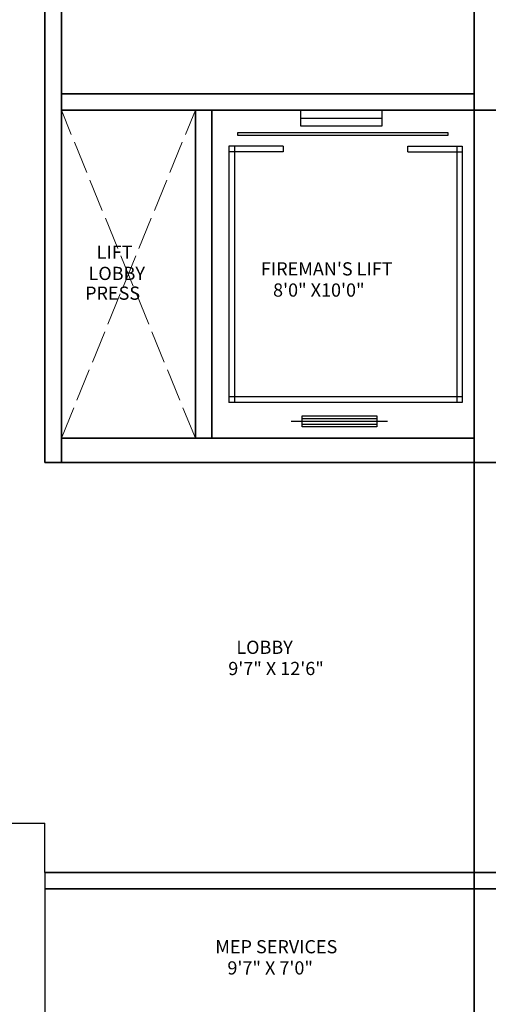
# Model space of a CAD drawing. Units: inches. Extents: x -61 to 1599, y -1316 to 257.
# Tile 161 of 204: x 826 to 998, y -939 to -579. Entities that reach past the tile are written whole.
import ezdxf

# ---------------------------------------------------------------- set-up
doc = ezdxf.new("R2010")
doc.units = ezdxf.units.IN
doc.header["$MEASUREMENT"] = 0
doc.linetypes.add('ACAD_ISO02W100', pattern=[15, 12, -3])
for name, color, linetype, lineweight in [('A-AREA-IDEN', 1, 'Continuous', 18), ('A-EQPM-ELEV', 150, 'Continuous', 25), ('A-FLOR-OPEN-HIDN', 8, 'ACAD_ISO02W100', 13), ('A-FLOR-STRS', 8, 'Continuous', 25), ('WALLS', 4, 'Continuous', 35)]:
    doc.layers.add(name, color=color, linetype=linetype, lineweight=lineweight)
doc.styles.get("Standard").update_dxf_attribs({"font": 'arial.ttf'})

msp = doc.modelspace()

# ---------------------------------------------------------------- linework, layer by layer
at = {"layer": 'A-EQPM-ELEV'}
for p, q in [((929.2181, -615.1047), (958.9007, -615.1047)), ((922.8184, -625.3496), (902.9834, -625.3496)), ((902.9834, -625.3496), (902.9834, -719.133)), ((904.9834, -625.3496), (904.9834, -719.133)), ((922.8184, -625.3496), (922.8184, -627.3496)), ((968.4601, -625.3496), (988.2951, -625.3496)), ((968.4601, -627.3496), (968.4601, -625.3496)), ((986.2951, -625.3496), (986.2951, -719.133)), ((988.2951, -625.3496), (988.2951, -719.133)), ((922.8184, -627.3496), (902.9834, -627.3496)), ((968.4601, -627.3496), (988.2951, -627.3496)), ((988.2951, -717.133), (902.9834, -717.133)), ((988.2951, -719.133), (902.9834, -719.133)), ((925.7144, -726.0279), (929.7123, -726.0279)), ((929.7123, -725.0279), (957.0257, -725.0279)), ((929.7123, -726.0279), (957.0257, -726.0279)), ((929.7123, -727.0279), (957.0257, -727.0279)), ((957.0257, -726.0279), (961.0237, -726.0279))]:
    msp.add_line(p, q, dxfattribs=at)
for points in [[(958.9007, -618.0403), (929.2181, -618.0403), (929.2181, -612.169), (958.9007, -612.169)], [(983.0641, -621.4772), (906.2073, -621.4772), (906.2073, -620.2665), (983.0641, -620.2665)], [(957.0257, -728.0649), (929.7123, -728.0649), (929.7123, -723.9909), (957.0257, -723.9909)]]:
    msp.add_lwpolyline(points, close=True, dxfattribs=at)
at = {"layer": 'A-FLOR-OPEN-HIDN'}
for p, q in [((841.7028, -732.169), (890.7028, -612.169)), ((890.7028, -732.169), (841.7028, -612.169))]:
    msp.add_line(p, q, dxfattribs=at)
at = {"layer": 'A-FLOR-STRS'}
for p, q in [((823.7028, -873.169), (835.7028, -873.169)), ((835.7028, -891.169), (835.7028, -873.169)), ((835.7028, -891.169), (835.7028, -1178.7933))]:
    msp.add_line(p, q, dxfattribs=at)
at = {"layer": 'WALLS'}
for p, q in [((835.7028, -61.169), (835.7028, -741.169)), ((841.7028, -61.169), (841.7028, -612.169)), ((992.7028, -61.169), (992.7028, -612.169)), ((992.7028, -606.169), (841.7028, -606.169)), ((992.7028, -612.169), (841.7028, -612.169)), ((841.7028, -732.169), (841.7028, -612.169)), ((890.7028, -732.169), (890.7028, -612.169)), ((896.7028, -732.169), (896.7028, -612.169)), ((992.7028, -741.169), (992.7028, -612.169)), ((1522.7028, -612.169), (992.7028, -612.169)), ((992.7028, -732.169), (841.7028, -732.169)), ((841.7028, -732.169), (841.7028, -741.169)), ((992.7028, -732.169), (992.7028, -741.169)), ((1001.7028, -741.169), (835.7028, -741.169)), ((992.7028, -1211.169), (992.7028, -741.169)), ((1001.7028, -891.169), (835.7028, -891.169)), ((1001.7028, -897.169), (835.7028, -897.169))]:
    msp.add_line(p, q, dxfattribs=at)

# ---------------------------------------------------------------- texts
at = {"layer": 'A-AREA-IDEN'}
for s, height, p in [('   LIFT', 4.8321, (850.1793, -666.5576)), (' LOBBY', 4.8321, (850.1793, -674.3199)), ("FIREMAN'S LIFT", 4.832098, (914.6942, -672.6471)), ('PRESS', 4.8321, (850.4048, -681.5506)), ('   8\'0" X10\'0"', 4.832098, (914.6942, -680.4095)), ('  LOBBY', 4.8321, (902.7455, -811.1806)), ('9\'7" X 12\'6"', 4.832098, (902.7455, -818.9429)), ('MEP SERVICES', 4.832098, (898.0015, -920.7792)), ('   9\'7" X 7\'0"', 4.832098, (898.0015, -928.5415))]:
    msp.add_text(s, height=height, dxfattribs=at).set_placement(p)

doc.saveas('drawing.dxf')
